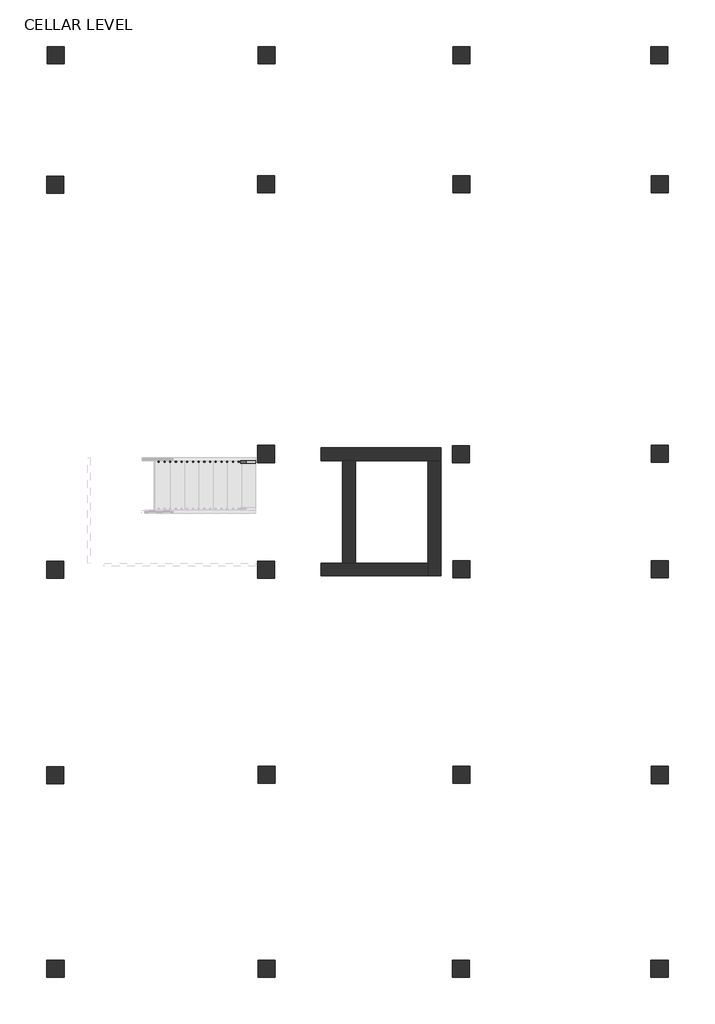
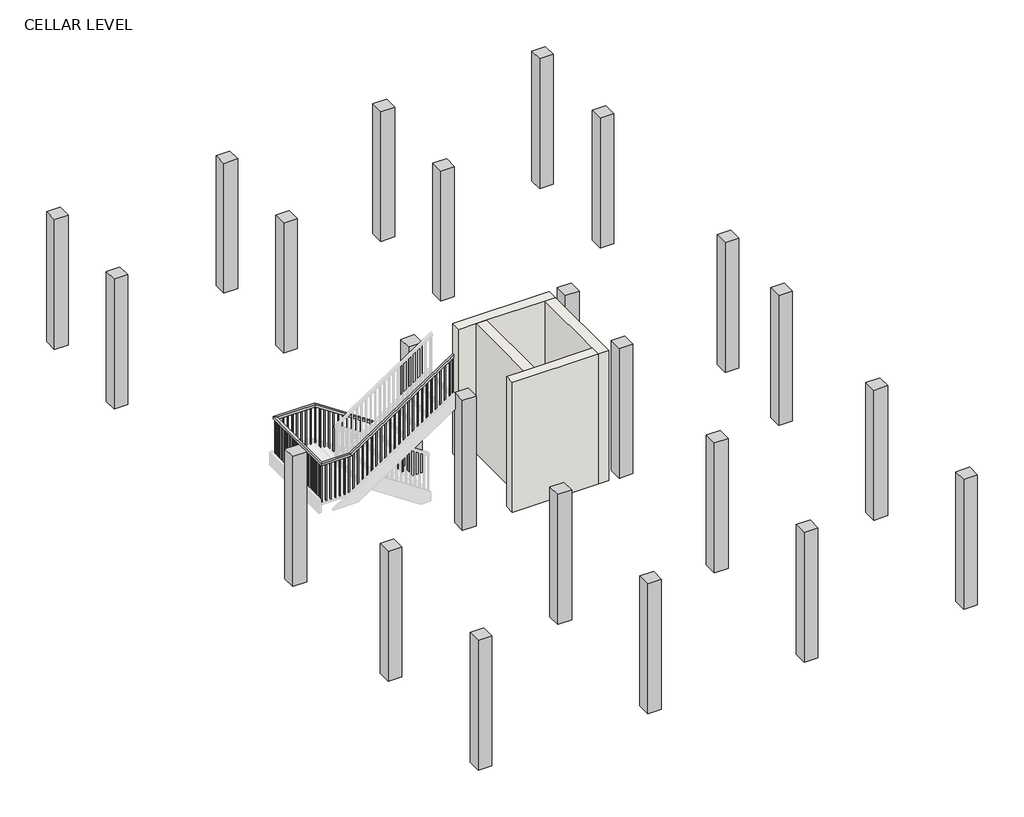
# One storey, part 1 of 2: 23 columns, 4 walls, 1 railing.
"""IFC4 building model written with IfcOpenShell, lengths in millimetres."""

from ifc_helpers import new_model, si_unit, frame, origin, origin_with_axes, place, context, project, spatial, polyline, outline, extrude, faceted_brep, transform, mapped, element, save
from components import rectangular_column_1_x_1_column_d780e21f

model = new_model("IFC4")

# Units and contexts
model_context = context("Model", 3, world=origin())
ifc_project = project(units=[si_unit("LENGTHUNIT", "METRE", prefix="MILLI")], contexts=[model_context])

# Site, building, storey
site = spatial("IfcSite", under=ifc_project)
building = spatial("IfcBuilding", under=site)
storey = spatial("IfcBuildingStorey", under=building, Name="CELLAR LEVEL", Elevation=0.0)

# Columns
placement = place(None, origin())
rectangular_column_1_x_1_column_shape = rectangular_column_1_x_1_column_d780e21f(model_context)
element("IfcColumn", 1, ObjectType="Rectangular Column : 1' X 1' COLUMN", at=placement, inside=storey, context=model_context, shape_type="MappedRepresentation", body=[
    mapped(rectangular_column_1_x_1_column_shape, transform((-6315.4590553, 13154.2270478, 0.0), x_axis=(1.0, 0.0, 0.0), y_axis=(0.0, 1.0, 0.0), z_axis=(0.0, 0.0, 1.0))),
])
element("IfcColumn", 2, ObjectType="Rectangular Column : 1' X 1' COLUMN", at=placement, inside=storey, context=model_context, shape_type="MappedRepresentation", body=[
    mapped(rectangular_column_1_x_1_column_shape, transform((-2556.0662097, 13154.2270478, 0.0), x_axis=(1.0, 0.0, 0.0), y_axis=(0.0, 1.0, 0.0), z_axis=(0.0, 0.0, 1.0))),
])
element("IfcColumn", 3, ObjectType="Rectangular Column : 1' X 1' COLUMN", at=placement, inside=storey, context=model_context, shape_type="MappedRepresentation", body=[
    mapped(rectangular_column_1_x_1_column_shape, transform((923.3718495, 13154.2270478, 0.0), x_axis=(1.0, 0.0, 0.0), y_axis=(0.0, 1.0, 0.0), z_axis=(0.0, 0.0, 1.0))),
])
element("IfcColumn", 4, ObjectType="Rectangular Column : 1' X 1' COLUMN", at=placement, inside=storey, context=model_context, shape_type="MappedRepresentation", body=[
    mapped(rectangular_column_1_x_1_column_shape, transform((-6323.7986459, 10846.022018, 0.0), x_axis=(1.0, 0.0, 0.0), y_axis=(0.0, 1.0, 0.0), z_axis=(0.0, 0.0, 1.0))),
])
element("IfcColumn", 5, ObjectType="Rectangular Column : 1' X 1' COLUMN", at=placement, inside=storey, context=model_context, shape_type="MappedRepresentation", body=[
    mapped(rectangular_column_1_x_1_column_shape, transform((-2562.3933654, 10852.5195509, 0.0), x_axis=(1.0, 0.0, 0.0), y_axis=(0.0, 1.0, 0.0), z_axis=(0.0, 0.0, 1.0))),
])
element("IfcColumn", 6, ObjectType="Rectangular Column : 1' X 1' COLUMN", at=placement, inside=storey, context=model_context, shape_type="MappedRepresentation", body=[
    mapped(rectangular_column_1_x_1_column_shape, transform((923.3718495, 10852.5195509, 0.0), x_axis=(1.0, 0.0, 0.0), y_axis=(0.0, 1.0, 0.0), z_axis=(0.0, 0.0, 1.0))),
])
element("IfcColumn", 7, ObjectType="Rectangular Column : 1' X 1' COLUMN", at=placement, inside=storey, context=model_context, shape_type="MappedRepresentation", body=[
    mapped(rectangular_column_1_x_1_column_shape, transform((4456.6573447, 10852.5195509, 0.0), x_axis=(1.0, 0.0, 0.0), y_axis=(0.0, 1.0, 0.0), z_axis=(0.0, 0.0, 1.0))),
])
element("IfcColumn", 8, ObjectType="Rectangular Column : 1' X 1' COLUMN", at=placement, inside=storey, context=model_context, shape_type="MappedRepresentation", body=[
    mapped(rectangular_column_1_x_1_column_shape, transform((4445.1592017, 13154.2270478, 0.0), x_axis=(1.0, 0.0, 0.0), y_axis=(0.0, 1.0, 0.0), z_axis=(0.0, 0.0, 1.0))),
])
element("IfcColumn", 9, ObjectType="Rectangular Column : 1' X 1' COLUMN", at=placement, inside=storey, context=model_context, shape_type="MappedRepresentation", body=[
    mapped(rectangular_column_1_x_1_column_shape, transform((4457.7502249, 3991.7950133, 0.0), x_axis=(1.0, 0.0, 0.0), y_axis=(0.0, 1.0, 0.0), z_axis=(0.0, 0.0, 1.0))),
])
element("IfcColumn", 10, ObjectType="Rectangular Column : 1' X 1' COLUMN", at=placement, inside=storey, context=model_context, shape_type="MappedRepresentation", body=[
    mapped(rectangular_column_1_x_1_column_shape, transform((4454.8407745, 6048.4156854, 0.0), x_axis=(1.0, 0.0, 0.0), y_axis=(0.0, 1.0, 0.0), z_axis=(0.0, 0.0, 1.0))),
])
element("IfcColumn", 11, ObjectType="Rectangular Column : 1' X 1' COLUMN", at=placement, inside=storey, context=model_context, shape_type="MappedRepresentation", body=[
    mapped(rectangular_column_1_x_1_column_shape, transform((909.0918469, 6040.7269851, 0.0), x_axis=(1.0, 0.0, 0.0), y_axis=(0.0, 1.0, 0.0), z_axis=(0.0, 0.0, 1.0))),
])
element("IfcColumn", 12, ObjectType="Rectangular Column : 1' X 1' COLUMN", at=placement, inside=storey, context=model_context, shape_type="MappedRepresentation", body=[
    mapped(rectangular_column_1_x_1_column_shape, transform((919.4097457, 3991.7950133, 0.0), x_axis=(1.0, 0.0, 0.0), y_axis=(0.0, 1.0, 0.0), z_axis=(0.0, 0.0, 1.0))),
])
element("IfcColumn", 13, ObjectType="Rectangular Column : 1' X 1' COLUMN", at=placement, inside=storey, context=model_context, shape_type="MappedRepresentation", body=[
    mapped(rectangular_column_1_x_1_column_shape, transform((-2560.9256766, 3983.754581, 0.0), x_axis=(1.0, 0.0, 0.0), y_axis=(0.0, 1.0, 0.0), z_axis=(0.0, 0.0, 1.0))),
])
element("IfcColumn", 14, ObjectType="Rectangular Column : 1' X 1' COLUMN", at=placement, inside=storey, context=model_context, shape_type="MappedRepresentation", body=[
    mapped(rectangular_column_1_x_1_column_shape, transform((-2562.176303, 6047.2663566, 0.0), x_axis=(1.0, 0.0, 0.0), y_axis=(0.0, 1.0, 0.0), z_axis=(0.0, 0.0, 1.0))),
])
element("IfcColumn", 15, ObjectType="Rectangular Column : 1' X 1' COLUMN", at=placement, inside=storey, context=model_context, shape_type="MappedRepresentation", body=[
    mapped(rectangular_column_1_x_1_column_shape, transform((-6324.6302424, 3983.0441655, 0.0), x_axis=(1.0, 0.0, 0.0), y_axis=(0.0, 1.0, 0.0), z_axis=(0.0, 0.0, 1.0))),
])
element("IfcColumn", 16, ObjectType="Rectangular Column : 1' X 1' COLUMN", at=placement, inside=storey, context=model_context, shape_type="MappedRepresentation", body=[
    mapped(rectangular_column_1_x_1_column_shape, transform((-6324.9283056, 323.449185, 0.0), x_axis=(1.0, 0.0, 0.0), y_axis=(0.0, 1.0, 0.0), z_axis=(0.0, 0.0, 1.0))),
])
element("IfcColumn", 17, ObjectType="Rectangular Column : 1' X 1' COLUMN", at=placement, inside=storey, context=model_context, shape_type="MappedRepresentation", body=[
    mapped(rectangular_column_1_x_1_column_shape, transform((-2552.5843312, 335.2664288, 0.0), x_axis=(1.0, 0.0, 0.0), y_axis=(0.0, 1.0, 0.0), z_axis=(0.0, 0.0, 1.0))),
])
element("IfcColumn", 18, ObjectType="Rectangular Column : 1' X 1' COLUMN", at=placement, inside=storey, context=model_context, shape_type="MappedRepresentation", body=[
    mapped(rectangular_column_1_x_1_column_shape, transform((919.1872547, 331.5602318, 0.0), x_axis=(1.0, 0.0, 0.0), y_axis=(0.0, 1.0, 0.0), z_axis=(0.0, 0.0, 1.0))),
])
element("IfcColumn", 19, ObjectType="Rectangular Column : 1' X 1' COLUMN", at=placement, inside=storey, context=model_context, shape_type="MappedRepresentation", body=[
    mapped(rectangular_column_1_x_1_column_shape, transform((4454.2172993, 328.0325771, 0.0), x_axis=(1.0, 0.0, 0.0), y_axis=(0.0, 1.0, 0.0), z_axis=(0.0, 0.0, 1.0))),
])
element("IfcColumn", 20, ObjectType="Rectangular Column : 1' X 1' COLUMN", at=placement, inside=storey, context=model_context, shape_type="MappedRepresentation", body=[
    mapped(rectangular_column_1_x_1_column_shape, transform((4452.0029555, -3126.4227345, 0.0), x_axis=(1.0, 0.0, 0.0), y_axis=(0.0, 1.0, 0.0), z_axis=(0.0, 0.0, 1.0))),
])
element("IfcColumn", 21, ObjectType="Rectangular Column : 1' X 1' COLUMN", at=placement, inside=storey, context=model_context, shape_type="MappedRepresentation", body=[
    mapped(rectangular_column_1_x_1_column_shape, transform((914.5144591, -3126.4227345, 0.0), x_axis=(1.0, 0.0, 0.0), y_axis=(0.0, 1.0, 0.0), z_axis=(0.0, 0.0, 1.0))),
])
element("IfcColumn", 22, ObjectType="Rectangular Column : 1' X 1' COLUMN", at=placement, inside=storey, context=model_context, shape_type="MappedRepresentation", body=[
    mapped(rectangular_column_1_x_1_column_shape, transform((-2553.2674339, -3121.3579443, 0.0), x_axis=(1.0, 0.0, 0.0), y_axis=(0.0, 1.0, 0.0), z_axis=(0.0, 0.0, 1.0))),
])
element("IfcColumn", 23, ObjectType="Rectangular Column : 1' X 1' COLUMN", at=placement, inside=storey, context=model_context, shape_type="MappedRepresentation", body=[
    mapped(rectangular_column_1_x_1_column_shape, transform((-6318.2578153, -3127.1571572, 0.0), x_axis=(1.0, 0.0, 0.0), y_axis=(0.0, 1.0, 0.0), z_axis=(0.0, 0.0, 1.0))),
])

# Railing
element("IfcRailing", 24, ObjectType="Handrail - Rectangular", at=placement, inside=storey, context=model_context, shape_type="SolidModel", body=[
    faceted_brep([(-2748.0012202, 5879.8309003, 1083.7333333), (-2748.0012202, 5879.8309003, 1022.6793317), (-2748.0012202, 5930.6309003, 1022.6793317), (-2748.0012202, 5930.6309003, 1083.7333333), (-4780.0012202, 5879.8309003, 2438.4), (-4795.3822226, 5879.8309003, 2387.6), (-4795.3822226, 5930.6309003, 2387.6), (-4780.0012202, 5930.6309003, 2438.4), (-5643.6012202, 5879.8309003, 2438.4), (-5643.6012202, 5879.8309003, 2387.6), (-5694.4012202, 5930.6309003, 2387.6), (-5694.4012202, 5930.6309003, 2438.4), (-5643.6012202, 4152.6309003, 2438.4), (-5643.6012202, 4152.6309003, 2387.6), (-5694.4012202, 4101.8309003, 2387.6), (-5694.4012202, 4101.8309003, 2438.4), (-5034.0012202, 4152.6309003, 2438.4), (-5018.6202178, 4152.6309003, 2387.6), (-5018.6202178, 4101.8309003, 2387.6), (-5034.0012202, 4101.8309003, 2438.4), (-2748.0012202, 4152.6309003, 3962.4), (-2748.0012202, 4101.8309003, 3962.4), (-2748.0012202, 4101.8309003, 3901.3459984), (-2748.0012202, 4152.6309003, 3901.3459984)], [[[0, 1, 2, 3]], [[1, 0, 4, 5]], [[2, 1, 5, 6]], [[3, 2, 6, 7]], [[0, 3, 7, 4]], [[5, 4, 8, 9]], [[6, 5, 9, 10]], [[7, 6, 10, 11]], [[4, 7, 11, 8]], [[9, 8, 12, 13]], [[10, 9, 13, 14]], [[11, 10, 14, 15]], [[8, 11, 15, 12]], [[13, 12, 16, 17]], [[14, 13, 17, 18]], [[15, 14, 18, 19]], [[12, 15, 19, 16]], [[20, 21, 22, 23]], [[17, 16, 20, 23]], [[18, 17, 23, 22]], [[19, 18, 22, 21]], [[16, 19, 21, 20]]]),
    extrude(outline(polyline([(3856.8959984, -2814.6762202), (3844.1959984, -2833.7262202), (2878.6666667, -2833.7262202), (2878.6666667, -2814.6762202), (3856.8959984, -2814.6762202)])), frame((0.0, 4117.7059003, 0.0), z_axis=(0.0, 1.0, 0.0), x_axis=(0.0, 0.0, 1.0)), (0.0, 0.0, 1.0), 19.05),
    extrude(outline(polyline([(3789.1626651, -2916.2762202), (3776.4626651, -2935.3262202), (2878.6666667, -2935.3262202), (2878.6666667, -2916.2762202), (3789.1626651, -2916.2762202)])), frame((0.0, 4117.7059003, 0.0), z_axis=(0.0, 1.0, 0.0), x_axis=(0.0, 0.0, 1.0)), (0.0, 0.0, 1.0), 19.05),
    extrude(outline(polyline([(3721.4293317, -3017.8762202), (3708.7293317, -3036.9262202), (2709.3333333, -3036.9262202), (2709.3333333, -3017.8762202), (3721.4293317, -3017.8762202)])), frame((0.0, 4117.7059003, 0.0), z_axis=(0.0, 1.0, 0.0), x_axis=(0.0, 0.0, 1.0)), (0.0, 0.0, 1.0), 19.05),
    extrude(outline(polyline([(3653.6959984, -3119.4762202), (3640.9959984, -3138.5262202), (2709.3333333, -3138.5262202), (2709.3333333, -3119.4762202), (3653.6959984, -3119.4762202)])), frame((0.0, 4117.7059003, 0.0), z_axis=(0.0, 1.0, 0.0), x_axis=(0.0, 0.0, 1.0)), (0.0, 0.0, 1.0), 19.05),
    extrude(outline(polyline([(3585.9626651, -3221.0762202), (3573.2626651, -3240.1262202), (2709.3333333, -3240.1262202), (2709.3333333, -3221.0762202), (3585.9626651, -3221.0762202)])), frame((0.0, 4117.7059003, 0.0), z_axis=(0.0, 1.0, 0.0), x_axis=(0.0, 0.0, 1.0)), (0.0, 0.0, 1.0), 19.05),
    extrude(outline(polyline([(3518.2293317, -3322.6762202), (3505.5293317, -3341.7262202), (2540.0, -3341.7262202), (2540.0, -3322.6762202), (3518.2293317, -3322.6762202)])), frame((0.0, 4117.7059003, 0.0), z_axis=(0.0, 1.0, 0.0), x_axis=(0.0, 0.0, 1.0)), (0.0, 0.0, 1.0), 19.05),
    extrude(outline(polyline([(3450.4959984, -3424.2762202), (3437.7959984, -3443.3262202), (2540.0, -3443.3262202), (2540.0, -3424.2762202), (3450.4959984, -3424.2762202)])), frame((0.0, 4117.7059003, 0.0), z_axis=(0.0, 1.0, 0.0), x_axis=(0.0, 0.0, 1.0)), (0.0, 0.0, 1.0), 19.05),
    extrude(outline(polyline([(3382.7626651, -3525.8762202), (3370.0626651, -3544.9262202), (2370.6666667, -3544.9262202), (2370.6666667, -3525.8762202), (3382.7626651, -3525.8762202)])), frame((0.0, 4117.7059003, 0.0), z_axis=(0.0, 1.0, 0.0), x_axis=(0.0, 0.0, 1.0)), (0.0, 0.0, 1.0), 19.05),
    extrude(outline(polyline([(3315.0293317, -3627.4762202), (3302.3293317, -3646.5262202), (2370.6666667, -3646.5262202), (2370.6666667, -3627.4762202), (3315.0293317, -3627.4762202)])), frame((0.0, 4117.7059003, 0.0), z_axis=(0.0, 1.0, 0.0), x_axis=(0.0, 0.0, 1.0)), (0.0, 0.0, 1.0), 19.05),
    extrude(outline(polyline([(3247.2959984, -3729.0762202), (3234.5959984, -3748.1262202), (2370.6666667, -3748.1262202), (2370.6666667, -3729.0762202), (3247.2959984, -3729.0762202)])), frame((0.0, 4117.7059003, 0.0), z_axis=(0.0, 1.0, 0.0), x_axis=(0.0, 0.0, 1.0)), (0.0, 0.0, 1.0), 19.05),
    extrude(outline(polyline([(3179.5626651, -3830.6762202), (3166.8626651, -3849.7262202), (2201.3333333, -3849.7262202), (2201.3333333, -3830.6762202), (3179.5626651, -3830.6762202)])), frame((0.0, 4117.7059003, 0.0), z_axis=(0.0, 1.0, 0.0), x_axis=(0.0, 0.0, 1.0)), (0.0, 0.0, 1.0), 19.05),
    extrude(outline(polyline([(3111.8293317, -3932.2762202), (3099.1293317, -3951.3262202), (2201.3333333, -3951.3262202), (2201.3333333, -3932.2762202), (3111.8293317, -3932.2762202)])), frame((0.0, 4117.7059003, 0.0), z_axis=(0.0, 1.0, 0.0), x_axis=(0.0, 0.0, 1.0)), (0.0, 0.0, 1.0), 19.05),
    extrude(outline(polyline([(3044.0959984, -4033.8762202), (3031.3959984, -4052.9262202), (2032.0, -4052.9262202), (2032.0, -4033.8762202), (3044.0959984, -4033.8762202)])), frame((0.0, 4117.7059003, 0.0), z_axis=(0.0, 1.0, 0.0), x_axis=(0.0, 0.0, 1.0)), (0.0, 0.0, 1.0), 19.05),
    extrude(outline(polyline([(2976.3626651, -4135.4762202), (2963.6626651, -4154.5262202), (2032.0, -4154.5262202), (2032.0, -4135.4762202), (2976.3626651, -4135.4762202)])), frame((0.0, 4117.7059003, 0.0), z_axis=(0.0, 1.0, 0.0), x_axis=(0.0, 0.0, 1.0)), (0.0, 0.0, 1.0), 19.05),
    extrude(outline(polyline([(2908.6293317, -4237.0762202), (2895.9293317, -4256.1262202), (2032.0, -4256.1262202), (2032.0, -4237.0762202), (2908.6293317, -4237.0762202)])), frame((0.0, 4117.7059003, 0.0), z_axis=(0.0, 1.0, 0.0), x_axis=(0.0, 0.0, 1.0)), (0.0, 0.0, 1.0), 19.05),
    extrude(outline(polyline([(2840.8959984, -4338.6762202), (2828.1959984, -4357.7262202), (1862.6666667, -4357.7262202), (1862.6666667, -4338.6762202), (2840.8959984, -4338.6762202)])), frame((0.0, 4117.7059003, 0.0), z_axis=(0.0, 1.0, 0.0), x_axis=(0.0, 0.0, 1.0)), (0.0, 0.0, 1.0), 19.05),
    extrude(outline(polyline([(2773.1626651, -4440.2762202), (2760.4626651, -4459.3262202), (1862.6666667, -4459.3262202), (1862.6666667, -4440.2762202), (2773.1626651, -4440.2762202)])), frame((0.0, 4117.7059003, 0.0), z_axis=(0.0, 1.0, 0.0), x_axis=(0.0, 0.0, 1.0)), (0.0, 0.0, 1.0), 19.05),
    extrude(outline(polyline([(2705.4293317, -4541.8762202), (2692.7293317, -4560.9262202), (1693.3333333, -4560.9262202), (1693.3333333, -4541.8762202), (2705.4293317, -4541.8762202)])), frame((0.0, 4117.7059003, 0.0), z_axis=(0.0, 1.0, 0.0), x_axis=(0.0, 0.0, 1.0)), (0.0, 0.0, 1.0), 19.05),
    extrude(outline(polyline([(2637.6959984, -4643.4762202), (2624.9959984, -4662.5262202), (1693.3333333, -4662.5262202), (1693.3333333, -4643.4762202), (2637.6959984, -4643.4762202)])), frame((0.0, 4117.7059003, 0.0), z_axis=(0.0, 1.0, 0.0), x_axis=(0.0, 0.0, 1.0)), (0.0, 0.0, 1.0), 19.05),
    extrude(outline(polyline([(2569.9626651, -4745.0762202), (2557.2626651, -4764.1262202), (1693.3333333, -4764.1262202), (1693.3333333, -4745.0762202), (2569.9626651, -4745.0762202)])), frame((0.0, 4117.7059003, 0.0), z_axis=(0.0, 1.0, 0.0), x_axis=(0.0, 0.0, 1.0)), (0.0, 0.0, 1.0), 19.05),
    extrude(outline(polyline([(2502.2293317, -4846.6762202), (2489.5293317, -4865.7262202), (1524.0, -4865.7262202), (1524.0, -4846.6762202), (2502.2293317, -4846.6762202)])), frame((0.0, 4117.7059003, 0.0), z_axis=(0.0, 1.0, 0.0), x_axis=(0.0, 0.0, 1.0)), (0.0, 0.0, 1.0), 19.05),
    extrude(outline(polyline([(2434.4959984, -4948.2762202), (2421.7959984, -4967.3262202), (1524.0, -4967.3262202), (1524.0, -4948.2762202), (2434.4959984, -4948.2762202)])), frame((0.0, 4117.7059003, 0.0), z_axis=(0.0, 1.0, 0.0), x_axis=(0.0, 0.0, 1.0)), (0.0, 0.0, 1.0), 19.05),
    extrude(outline(polyline([(-5068.9262202, 4117.7059003), (-5068.9262202, 4136.7559003), (-5049.8762202, 4136.7559003), (-5049.8762202, 4117.7059003), (-5068.9262202, 4117.7059003)])), frame((0.0, 0.0, 1524.0), z_axis=(0.0, 0.0, 1.0), x_axis=(1.0, 0.0, 0.0)), (0.0, 0.0, 1.0), 863.6),
    extrude(outline(polyline([(-5170.5262202, 4117.7059003), (-5170.5262202, 4136.7559003), (-5151.4762202, 4136.7559003), (-5151.4762202, 4117.7059003), (-5170.5262202, 4117.7059003)])), frame((0.0, 0.0, 1524.0), z_axis=(0.0, 0.0, 1.0), x_axis=(1.0, 0.0, 0.0)), (0.0, 0.0, 1.0), 863.6),
    extrude(outline(polyline([(-5272.1262202, 4117.7059003), (-5272.1262202, 4136.7559003), (-5253.0762202, 4136.7559003), (-5253.0762202, 4117.7059003), (-5272.1262202, 4117.7059003)])), frame((0.0, 0.0, 1524.0), z_axis=(0.0, 0.0, 1.0), x_axis=(1.0, 0.0, 0.0)), (0.0, 0.0, 1.0), 863.6),
    extrude(outline(polyline([(-5373.7262202, 4117.7059003), (-5373.7262202, 4136.7559003), (-5354.6762202, 4136.7559003), (-5354.6762202, 4117.7059003), (-5373.7262202, 4117.7059003)])), frame((0.0, 0.0, 1524.0), z_axis=(0.0, 0.0, 1.0), x_axis=(1.0, 0.0, 0.0)), (0.0, 0.0, 1.0), 863.6),
    extrude(outline(polyline([(-5475.3262202, 4117.7059003), (-5475.3262202, 4136.7559003), (-5456.2762202, 4136.7559003), (-5456.2762202, 4117.7059003), (-5475.3262202, 4117.7059003)])), frame((0.0, 0.0, 1524.0), z_axis=(0.0, 0.0, 1.0), x_axis=(1.0, 0.0, 0.0)), (0.0, 0.0, 1.0), 863.6),
    extrude(outline(polyline([(-5576.9262202, 4117.7059003), (-5576.9262202, 4136.7559003), (-5557.8762202, 4136.7559003), (-5557.8762202, 4117.7059003), (-5576.9262202, 4117.7059003)])), frame((0.0, 0.0, 1524.0), z_axis=(0.0, 0.0, 1.0), x_axis=(1.0, 0.0, 0.0)), (0.0, 0.0, 1.0), 863.6),
    extrude(outline(polyline([(-5678.5262202, 4187.5559003), (-5659.4762202, 4187.5559003), (-5659.4762202, 4168.5059003), (-5678.5262202, 4168.5059003), (-5678.5262202, 4187.5559003)])), frame((0.0, 0.0, 1524.0), z_axis=(0.0, 0.0, 1.0), x_axis=(1.0, 0.0, 0.0)), (0.0, 0.0, 1.0), 863.6),
    extrude(outline(polyline([(-5678.5262202, 4289.1559003), (-5659.4762202, 4289.1559003), (-5659.4762202, 4270.1059003), (-5678.5262202, 4270.1059003), (-5678.5262202, 4289.1559003)])), frame((0.0, 0.0, 1524.0), z_axis=(0.0, 0.0, 1.0), x_axis=(1.0, 0.0, 0.0)), (0.0, 0.0, 1.0), 863.6),
    extrude(outline(polyline([(-5678.5262202, 4390.7559003), (-5659.4762202, 4390.7559003), (-5659.4762202, 4371.7059003), (-5678.5262202, 4371.7059003), (-5678.5262202, 4390.7559003)])), frame((0.0, 0.0, 1524.0), z_axis=(0.0, 0.0, 1.0), x_axis=(1.0, 0.0, 0.0)), (0.0, 0.0, 1.0), 863.6),
    extrude(outline(polyline([(-5678.5262202, 4492.3559003), (-5659.4762202, 4492.3559003), (-5659.4762202, 4473.3059003), (-5678.5262202, 4473.3059003), (-5678.5262202, 4492.3559003)])), frame((0.0, 0.0, 1524.0), z_axis=(0.0, 0.0, 1.0), x_axis=(1.0, 0.0, 0.0)), (0.0, 0.0, 1.0), 863.6),
    extrude(outline(polyline([(-5678.5262202, 4593.9559003), (-5659.4762202, 4593.9559003), (-5659.4762202, 4574.9059003), (-5678.5262202, 4574.9059003), (-5678.5262202, 4593.9559003)])), frame((0.0, 0.0, 1524.0), z_axis=(0.0, 0.0, 1.0), x_axis=(1.0, 0.0, 0.0)), (0.0, 0.0, 1.0), 863.6),
    extrude(outline(polyline([(-5678.5262202, 4695.5559003), (-5659.4762202, 4695.5559003), (-5659.4762202, 4676.5059003), (-5678.5262202, 4676.5059003), (-5678.5262202, 4695.5559003)])), frame((0.0, 0.0, 1524.0), z_axis=(0.0, 0.0, 1.0), x_axis=(1.0, 0.0, 0.0)), (0.0, 0.0, 1.0), 863.6),
    extrude(outline(polyline([(-5678.5262202, 4797.1559003), (-5659.4762202, 4797.1559003), (-5659.4762202, 4778.1059003), (-5678.5262202, 4778.1059003), (-5678.5262202, 4797.1559003)])), frame((0.0, 0.0, 1524.0), z_axis=(0.0, 0.0, 1.0), x_axis=(1.0, 0.0, 0.0)), (0.0, 0.0, 1.0), 863.6),
    extrude(outline(polyline([(-5678.5262202, 4898.7559003), (-5659.4762202, 4898.7559003), (-5659.4762202, 4879.7059003), (-5678.5262202, 4879.7059003), (-5678.5262202, 4898.7559003)])), frame((0.0, 0.0, 1524.0), z_axis=(0.0, 0.0, 1.0), x_axis=(1.0, 0.0, 0.0)), (0.0, 0.0, 1.0), 863.6),
    extrude(outline(polyline([(-5678.5262202, 5000.3559003), (-5659.4762202, 5000.3559003), (-5659.4762202, 4981.3059003), (-5678.5262202, 4981.3059003), (-5678.5262202, 5000.3559003)])), frame((0.0, 0.0, 1524.0), z_axis=(0.0, 0.0, 1.0), x_axis=(1.0, 0.0, 0.0)), (0.0, 0.0, 1.0), 863.6),
    extrude(outline(polyline([(-5678.5262202, 5101.9559003), (-5659.4762202, 5101.9559003), (-5659.4762202, 5082.9059003), (-5678.5262202, 5082.9059003), (-5678.5262202, 5101.9559003)])), frame((0.0, 0.0, 1524.0), z_axis=(0.0, 0.0, 1.0), x_axis=(1.0, 0.0, 0.0)), (0.0, 0.0, 1.0), 863.6),
    extrude(outline(polyline([(-5678.5262202, 5203.5559003), (-5659.4762202, 5203.5559003), (-5659.4762202, 5184.5059003), (-5678.5262202, 5184.5059003), (-5678.5262202, 5203.5559003)])), frame((0.0, 0.0, 1524.0), z_axis=(0.0, 0.0, 1.0), x_axis=(1.0, 0.0, 0.0)), (0.0, 0.0, 1.0), 863.6),
    extrude(outline(polyline([(-5678.5262202, 5305.1559003), (-5659.4762202, 5305.1559003), (-5659.4762202, 5286.1059003), (-5678.5262202, 5286.1059003), (-5678.5262202, 5305.1559003)])), frame((0.0, 0.0, 1524.0), z_axis=(0.0, 0.0, 1.0), x_axis=(1.0, 0.0, 0.0)), (0.0, 0.0, 1.0), 863.6),
    extrude(outline(polyline([(-5678.5262202, 5406.7559003), (-5659.4762202, 5406.7559003), (-5659.4762202, 5387.7059003), (-5678.5262202, 5387.7059003), (-5678.5262202, 5406.7559003)])), frame((0.0, 0.0, 1524.0), z_axis=(0.0, 0.0, 1.0), x_axis=(1.0, 0.0, 0.0)), (0.0, 0.0, 1.0), 863.6),
    extrude(outline(polyline([(-5678.5262202, 5508.3559003), (-5659.4762202, 5508.3559003), (-5659.4762202, 5489.3059003), (-5678.5262202, 5489.3059003), (-5678.5262202, 5508.3559003)])), frame((0.0, 0.0, 1524.0), z_axis=(0.0, 0.0, 1.0), x_axis=(1.0, 0.0, 0.0)), (0.0, 0.0, 1.0), 863.6),
    extrude(outline(polyline([(-5678.5262202, 5609.9559003), (-5659.4762202, 5609.9559003), (-5659.4762202, 5590.9059003), (-5678.5262202, 5590.9059003), (-5678.5262202, 5609.9559003)])), frame((0.0, 0.0, 1524.0), z_axis=(0.0, 0.0, 1.0), x_axis=(1.0, 0.0, 0.0)), (0.0, 0.0, 1.0), 863.6),
    extrude(outline(polyline([(-5678.5262202, 5711.5559003), (-5659.4762202, 5711.5559003), (-5659.4762202, 5692.5059003), (-5678.5262202, 5692.5059003), (-5678.5262202, 5711.5559003)])), frame((0.0, 0.0, 1524.0), z_axis=(0.0, 0.0, 1.0), x_axis=(1.0, 0.0, 0.0)), (0.0, 0.0, 1.0), 863.6),
    extrude(outline(polyline([(-5678.5262202, 5813.1559003), (-5659.4762202, 5813.1559003), (-5659.4762202, 5794.1059003), (-5678.5262202, 5794.1059003), (-5678.5262202, 5813.1559003)])), frame((0.0, 0.0, 1524.0), z_axis=(0.0, 0.0, 1.0), x_axis=(1.0, 0.0, 0.0)), (0.0, 0.0, 1.0), 863.6),
    extrude(outline(polyline([(-5583.2762202, 5914.7559003), (-5583.2762202, 5895.7059003), (-5602.3262202, 5895.7059003), (-5602.3262202, 5914.7559003), (-5583.2762202, 5914.7559003)])), frame((0.0, 0.0, 1524.0), z_axis=(0.0, 0.0, 1.0), x_axis=(1.0, 0.0, 0.0)), (0.0, 0.0, 1.0), 863.6),
    extrude(outline(polyline([(-5481.6762202, 5914.7559003), (-5481.6762202, 5895.7059003), (-5500.7262202, 5895.7059003), (-5500.7262202, 5914.7559003), (-5481.6762202, 5914.7559003)])), frame((0.0, 0.0, 1524.0), z_axis=(0.0, 0.0, 1.0), x_axis=(1.0, 0.0, 0.0)), (0.0, 0.0, 1.0), 863.6),
    extrude(outline(polyline([(-5380.0762202, 5914.7559003), (-5380.0762202, 5895.7059003), (-5399.1262202, 5895.7059003), (-5399.1262202, 5914.7559003), (-5380.0762202, 5914.7559003)])), frame((0.0, 0.0, 1524.0), z_axis=(0.0, 0.0, 1.0), x_axis=(1.0, 0.0, 0.0)), (0.0, 0.0, 1.0), 863.6),
    extrude(outline(polyline([(-5278.4762202, 5914.7559003), (-5278.4762202, 5895.7059003), (-5297.5262202, 5895.7059003), (-5297.5262202, 5914.7559003), (-5278.4762202, 5914.7559003)])), frame((0.0, 0.0, 1524.0), z_axis=(0.0, 0.0, 1.0), x_axis=(1.0, 0.0, 0.0)), (0.0, 0.0, 1.0), 863.6),
    extrude(outline(polyline([(-5176.8762202, 5914.7559003), (-5176.8762202, 5895.7059003), (-5195.9262202, 5895.7059003), (-5195.9262202, 5914.7559003), (-5176.8762202, 5914.7559003)])), frame((0.0, 0.0, 1524.0), z_axis=(0.0, 0.0, 1.0), x_axis=(1.0, 0.0, 0.0)), (0.0, 0.0, 1.0), 863.6),
    extrude(outline(polyline([(-5075.2762202, 5914.7559003), (-5075.2762202, 5895.7059003), (-5094.3262202, 5895.7059003), (-5094.3262202, 5914.7559003), (-5075.2762202, 5914.7559003)])), frame((0.0, 0.0, 1524.0), z_axis=(0.0, 0.0, 1.0), x_axis=(1.0, 0.0, 0.0)), (0.0, 0.0, 1.0), 863.6),
    extrude(outline(polyline([(-4973.6762202, 5914.7559003), (-4973.6762202, 5895.7059003), (-4992.7262202, 5895.7059003), (-4992.7262202, 5914.7559003), (-4973.6762202, 5914.7559003)])), frame((0.0, 0.0, 1524.0), z_axis=(0.0, 0.0, 1.0), x_axis=(1.0, 0.0, 0.0)), (0.0, 0.0, 1.0), 863.6),
    extrude(outline(polyline([(-4872.0762202, 5914.7559003), (-4872.0762202, 5895.7059003), (-4891.1262202, 5895.7059003), (-4891.1262202, 5914.7559003), (-4872.0762202, 5914.7559003)])), frame((0.0, 0.0, 1524.0), z_axis=(0.0, 0.0, 1.0), x_axis=(1.0, 0.0, 0.0)), (0.0, 0.0, 1.0), 863.6),
    extrude(outline(polyline([(2370.9959984, -4770.4762202), (2383.6959984, -4789.5262202), (1524.0, -4789.5262202), (1524.0, -4770.4762202), (2370.9959984, -4770.4762202)])), frame((0.0, 5895.7059003, 0.0), z_axis=(0.0, 1.0, 0.0), x_axis=(0.0, 0.0, 1.0)), (0.0, 0.0, 1.0), 19.05),
    extrude(outline(polyline([(2303.2626651, -4668.8762202), (2315.9626651, -4687.9262202), (1354.6666667, -4687.9262202), (1354.6666667, -4668.8762202), (2303.2626651, -4668.8762202)])), frame((0.0, 5895.7059003, 0.0), z_axis=(0.0, 1.0, 0.0), x_axis=(0.0, 0.0, 1.0)), (0.0, 0.0, 1.0), 19.05),
    extrude(outline(polyline([(2235.5293317, -4567.2762202), (2248.2293317, -4586.3262202), (1354.6666667, -4586.3262202), (1354.6666667, -4567.2762202), (2235.5293317, -4567.2762202)])), frame((0.0, 5895.7059003, 0.0), z_axis=(0.0, 1.0, 0.0), x_axis=(0.0, 0.0, 1.0)), (0.0, 0.0, 1.0), 19.05),
    extrude(outline(polyline([(2167.7959984, -4465.6762202), (2180.4959984, -4484.7262202), (1185.3333333, -4484.7262202), (1185.3333333, -4465.6762202), (2167.7959984, -4465.6762202)])), frame((0.0, 5895.7059003, 0.0), z_axis=(0.0, 1.0, 0.0), x_axis=(0.0, 0.0, 1.0)), (0.0, 0.0, 1.0), 19.05),
    extrude(outline(polyline([(2100.0626651, -4364.0762202), (2112.7626651, -4383.1262202), (1185.3333333, -4383.1262202), (1185.3333333, -4364.0762202), (2100.0626651, -4364.0762202)])), frame((0.0, 5895.7059003, 0.0), z_axis=(0.0, 1.0, 0.0), x_axis=(0.0, 0.0, 1.0)), (0.0, 0.0, 1.0), 19.05),
    extrude(outline(polyline([(2032.3293317, -4262.4762202), (2045.0293317, -4281.5262202), (1185.3333333, -4281.5262202), (1185.3333333, -4262.4762202), (2032.3293317, -4262.4762202)])), frame((0.0, 5895.7059003, 0.0), z_axis=(0.0, 1.0, 0.0), x_axis=(0.0, 0.0, 1.0)), (0.0, 0.0, 1.0), 19.05),
    extrude(outline(polyline([(1964.5959984, -4160.8762202), (1977.2959984, -4179.9262202), (1016.0, -4179.9262202), (1016.0, -4160.8762202), (1964.5959984, -4160.8762202)])), frame((0.0, 5895.7059003, 0.0), z_axis=(0.0, 1.0, 0.0), x_axis=(0.0, 0.0, 1.0)), (0.0, 0.0, 1.0), 19.05),
    extrude(outline(polyline([(1896.8626651, -4059.2762202), (1909.5626651, -4078.3262202), (1016.0, -4078.3262202), (1016.0, -4059.2762202), (1896.8626651, -4059.2762202)])), frame((0.0, 5895.7059003, 0.0), z_axis=(0.0, 1.0, 0.0), x_axis=(0.0, 0.0, 1.0)), (0.0, 0.0, 1.0), 19.05),
    extrude(outline(polyline([(1829.1293317, -3957.6762202), (1841.8293317, -3976.7262202), (846.6666667, -3976.7262202), (846.6666667, -3957.6762202), (1829.1293317, -3957.6762202)])), frame((0.0, 5895.7059003, 0.0), z_axis=(0.0, 1.0, 0.0), x_axis=(0.0, 0.0, 1.0)), (0.0, 0.0, 1.0), 19.05),
    extrude(outline(polyline([(1761.3959984, -3856.0762202), (1774.0959984, -3875.1262202), (846.6666667, -3875.1262202), (846.6666667, -3856.0762202), (1761.3959984, -3856.0762202)])), frame((0.0, 5895.7059003, 0.0), z_axis=(0.0, 1.0, 0.0), x_axis=(0.0, 0.0, 1.0)), (0.0, 0.0, 1.0), 19.05),
    extrude(outline(polyline([(1693.6626651, -3754.4762202), (1706.3626651, -3773.5262202), (846.6666667, -3773.5262202), (846.6666667, -3754.4762202), (1693.6626651, -3754.4762202)])), frame((0.0, 5895.7059003, 0.0), z_axis=(0.0, 1.0, 0.0), x_axis=(0.0, 0.0, 1.0)), (0.0, 0.0, 1.0), 19.05),
    extrude(outline(polyline([(1625.9293317, -3652.8762202), (1638.6293317, -3671.9262202), (677.3333333, -3671.9262202), (677.3333333, -3652.8762202), (1625.9293317, -3652.8762202)])), frame((0.0, 5895.7059003, 0.0), z_axis=(0.0, 1.0, 0.0), x_axis=(0.0, 0.0, 1.0)), (0.0, 0.0, 1.0), 19.05),
    extrude(outline(polyline([(1558.1959984, -3551.2762202), (1570.8959984, -3570.3262202), (677.3333333, -3570.3262202), (677.3333333, -3551.2762202), (1558.1959984, -3551.2762202)])), frame((0.0, 5895.7059003, 0.0), z_axis=(0.0, 1.0, 0.0), x_axis=(0.0, 0.0, 1.0)), (0.0, 0.0, 1.0), 19.05),
    extrude(outline(polyline([(1490.4626651, -3449.6762202), (1503.1626651, -3468.7262202), (508.0, -3468.7262202), (508.0, -3449.6762202), (1490.4626651, -3449.6762202)])), frame((0.0, 5895.7059003, 0.0), z_axis=(0.0, 1.0, 0.0), x_axis=(0.0, 0.0, 1.0)), (0.0, 0.0, 1.0), 19.05),
    extrude(outline(polyline([(1422.7293317, -3348.0762202), (1435.4293317, -3367.1262202), (508.0, -3367.1262202), (508.0, -3348.0762202), (1422.7293317, -3348.0762202)])), frame((0.0, 5895.7059003, 0.0), z_axis=(0.0, 1.0, 0.0), x_axis=(0.0, 0.0, 1.0)), (0.0, 0.0, 1.0), 19.05),
    extrude(outline(polyline([(1354.9959984, -3246.4762202), (1367.6959984, -3265.5262202), (508.0, -3265.5262202), (508.0, -3246.4762202), (1354.9959984, -3246.4762202)])), frame((0.0, 5895.7059003, 0.0), z_axis=(0.0, 1.0, 0.0), x_axis=(0.0, 0.0, 1.0)), (0.0, 0.0, 1.0), 19.05),
    extrude(outline(polyline([(1287.2626651, -3144.8762202), (1299.9626651, -3163.9262202), (338.6666667, -3163.9262202), (338.6666667, -3144.8762202), (1287.2626651, -3144.8762202)])), frame((0.0, 5895.7059003, 0.0), z_axis=(0.0, 1.0, 0.0), x_axis=(0.0, 0.0, 1.0)), (0.0, 0.0, 1.0), 19.05),
    extrude(outline(polyline([(1219.5293317, -3043.2762202), (1232.2293317, -3062.3262202), (338.6666667, -3062.3262202), (338.6666667, -3043.2762202), (1219.5293317, -3043.2762202)])), frame((0.0, 5895.7059003, 0.0), z_axis=(0.0, 1.0, 0.0), x_axis=(0.0, 0.0, 1.0)), (0.0, 0.0, 1.0), 19.05),
    extrude(outline(polyline([(1151.7959984, -2941.6762202), (1164.4959984, -2960.7262202), (169.3333333, -2960.7262202), (169.3333333, -2941.6762202), (1151.7959984, -2941.6762202)])), frame((0.0, 5895.7059003, 0.0), z_axis=(0.0, 1.0, 0.0), x_axis=(0.0, 0.0, 1.0)), (0.0, 0.0, 1.0), 19.05),
    extrude(outline(polyline([(1084.0626651, -2840.0762202), (1096.7626651, -2859.1262202), (169.3333333, -2859.1262202), (169.3333333, -2840.0762202), (1084.0626651, -2840.0762202)])), frame((0.0, 5895.7059003, 0.0), z_axis=(0.0, 1.0, 0.0), x_axis=(0.0, 0.0, 1.0)), (0.0, 0.0, 1.0), 19.05),
    extrude(outline(polyline([(-5678.5262202, 4136.7559003), (-5659.4762202, 4136.7559003), (-5659.4762202, 4117.7059003), (-5678.5262202, 4117.7059003), (-5678.5262202, 4136.7559003)])), frame((0.0, 0.0, 1524.0), z_axis=(0.0, 0.0, 1.0), x_axis=(1.0, 0.0, 0.0)), (0.0, 0.0, 1.0), 863.6),
    extrude(outline(polyline([(-5659.4762202, 5914.7559003), (-5659.4762202, 5895.7059003), (-5678.5262202, 5895.7059003), (-5678.5262202, 5914.7559003), (-5659.4762202, 5914.7559003)])), frame((0.0, 0.0, 1524.0), z_axis=(0.0, 0.0, 1.0), x_axis=(1.0, 0.0, 0.0)), (0.0, 0.0, 1.0), 863.6),
    extrude(outline(polyline([(3901.3459984, -2748.0012202), (3888.6459984, -2767.0512202), (2878.6666667, -2767.0512202), (2878.6666667, -2748.0012202), (3901.3459984, -2748.0012202)])), frame((0.0, 4117.7059003, 0.0), z_axis=(0.0, 1.0, 0.0), x_axis=(0.0, 0.0, 1.0)), (0.0, 0.0, 1.0), 19.05),
    extrude(outline(polyline([(1022.6793317, -2748.0012202), (1035.3793317, -2767.0512202), (169.3333333, -2767.0512202), (169.3333333, -2748.0012202), (1022.6793317, -2748.0012202)])), frame((0.0, 5895.7059003, 0.0), z_axis=(0.0, 1.0, 0.0), x_axis=(0.0, 0.0, 1.0)), (0.0, 0.0, 1.0), 19.05),
])

# Walls
element("IfcWall", 25, ObjectType="OUTER WALL 9\"", at=placement, inside=storey, context=model_context, shape_type="Brep", body=[
    faceted_brep([(-1579.6012202, 5930.6309003, 0.0), (-1198.6012202, 5930.6309003, 0.0), (-970.0012202, 5930.6309003, 0.0), (325.3987798, 5930.6309003, 0.0), (553.9987798, 5930.6309003, 0.0), (553.9987798, 5930.6309003, 3048.0), (325.3987798, 5930.6309003, 3048.0), (-970.0012202, 5930.6309003, 3048.0), (-1198.6012202, 5930.6309003, 3048.0), (-1579.6012202, 5930.6309003, 3048.0), (-1579.6012202, 6159.2309003, 0.0), (-1579.6012202, 6159.2309003, 3048.0), (553.9987798, 6159.2309003, 3048.0), (553.9987798, 6159.2309003, 0.0)], [[[0, 1, 2, 3, 4, 5, 6, 7, 8, 9]], [[10, 11, 12, 13]], [[4, 3, 2, 1, 0, 10, 13]], [[9, 8, 7, 6, 5, 12, 11]], [[0, 9, 11, 10]], [[5, 4, 13, 12]]]),
])
element("IfcWall", 26, ObjectType="OUTER WALL 9\"", at=placement, inside=storey, context=model_context, shape_type="Brep", body=[
    faceted_brep([(325.3987798, 5930.6309003, 0.0), (325.3987798, 4101.8309003, 0.0), (325.3987798, 3873.2309003, 0.0), (325.3987798, 3873.2309003, 3048.0), (325.3987798, 4101.8309003, 3048.0), (325.3987798, 5930.6309003, 3048.0), (553.9987798, 5930.6309003, 0.0), (553.9987798, 5930.6309003, 3048.0), (553.9987798, 3873.2309003, 3048.0), (553.9987798, 3873.2309003, 0.0)], [[[0, 1, 2, 3, 4, 5]], [[6, 7, 8, 9]], [[2, 1, 0, 6, 9]], [[5, 4, 3, 8, 7]], [[0, 5, 7, 6]], [[3, 2, 9, 8]]]),
])
element("IfcWall", 27, ObjectType="OUTER WALL 9\"", at=placement, inside=storey, context=model_context, shape_type="Brep", body=[
    faceted_brep([(325.3987798, 4101.8309003, 0.0), (-970.0012202, 4101.8309003, 0.0), (-1198.6012202, 4101.8309003, 0.0), (-1579.6012202, 4101.8309003, 0.0), (-1579.6012202, 4101.8309003, 3048.0), (-1198.6012202, 4101.8309003, 3048.0), (-970.0012202, 4101.8309003, 3048.0), (325.3987798, 4101.8309003, 3048.0), (325.3987798, 3873.2309003, 0.0), (325.3987798, 3873.2309003, 3048.0), (-1579.6012202, 3873.2309003, 3048.0), (-1579.6012202, 3873.2309003, 0.0)], [[[0, 1, 2, 3, 4, 5, 6, 7]], [[8, 9, 10, 11]], [[3, 2, 1, 0, 8, 11]], [[4, 3, 11, 10]], [[7, 6, 5, 4, 10, 9]], [[0, 7, 9, 8]]]),
])
element("IfcWall", 28, ObjectType="OUTER WALL 9\"", at=placement, inside=storey, context=model_context, shape_type="SweptSolid", body=[
    extrude(outline(polyline([(-1198.6012202, 4101.8309003), (-1198.6012202, 5930.6309003), (-970.0012202, 5930.6309003), (-970.0012202, 4101.8309003), (-1198.6012202, 4101.8309003)])), origin_with_axes(), (0.0, 0.0, 1.0), 3048.0),
])

save(model, "model.ifc")

# Revit data of these elements
# Type "Rectangular Column : 1' X 1' COLUMN"
#   Assembly Code = "B1010200"
#   Depth = 1' - 0"
#   Offset Base = 0' - 0"
#   Offset Top = 0' - 0"
#   Width = 1' - 0"
#   Material = ROSE COLOUR
# Type "Handrail - Rectangular"
#   Assembly Code = "C2010400"
#   built-in parameter 1008612 = 0.0416667 (stored number, unit not read)
#   built-in parameter 1008611 = 0.0416667 (stored number, unit not read)
#   built-in parameter 1008609 = 0.333333 (stored number, unit not read)
#   built-in parameter 1008604 = 0.166667 (stored number, unit not read)
#   built-in parameter 1008603 = 0.166667 (stored number, unit not read)
#   Railing Height = 3' - 0"
#   built-in parameter 1008630 = 2
#   built-in parameter 1008610 = 2
#   built-in parameter 1008618 = Baluster - Square : 3/4"
# Type "OUTER WALL 9\""
#   Assembly Code = "B2010"
#   Layers, outside or top first: 0' - 9" "ROSE COLOUR" (function 1)
# Elements 1, 2, 3, 4, 5, 6, 7, 8, 9, 10, 11, 12, 13, 14, 15, 16, 17, 18, 19, 20, 21, 22, 23 (IfcColumn, "Rectangular Column : 1' X 1' COLUMN")
#   Phase Created = New Construction
#   Materials on its faces: "ROSE COLOUR"
# Element 24 (IfcRailing, "Handrail - Rectangular")
#   Phase Created = New Construction
# Elements 25, 26, 27, 28 (IfcWall, "OUTER WALL 9\"")
#   Top Offset = 0' - 0"
#   Base Offset = 0' - 0"
#   wall height = 10' - 0"
#   Phase Created = New Construction
#   Base Constraint = CELLAR LEVEL
#   Top Constraint = GROUND LVL
#   Materials on its faces: "ROSE COLOUR"
# Materials
#   "ROSE COLOUR": class "Generic", colour RGB 120 120 120, transparency 0, Cost = 0
